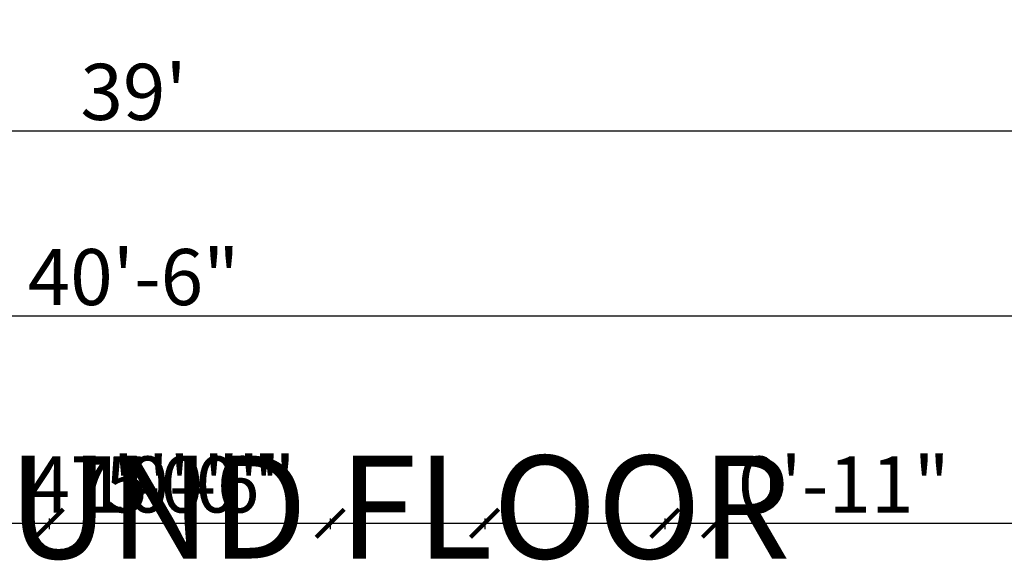
# Model space of a CAD drawing. Units: inches. Extents: x 261 to 2725, y 291 to 1454.
# Tile 7 of 35: x 688 to 898, y 296 to 412. Entities that reach past the tile are written whole.
import ezdxf

# ---------------------------------------------------------------- set-up
doc = ezdxf.new("R2010")
doc.units = ezdxf.units.IN
doc.layers.add('A-ANNO-DIMS', color=136, linetype='Continuous', lineweight=18)
doc.layers.add('A-ANNO-TEXT', color=7, linetype='Continuous', lineweight=25)
doc.styles.get("Standard").update_dxf_attribs({"font": 'arial.ttf'})
doc.dimstyles.new('ISO-25', dxfattribs={"dimtxt": 12, "dimasz": 6, "dimexe": 1.25, "dimexo": 0.625, "dimtad": 1, "dimdec": 0, "dimlunit": 3, "dimtxsty": 'Standard', "dimblk": 'ARCHTICK', "dimcen": 2.5, "dimadec": 0, "dimazin": 0, "dimtfac": 1, "dimtdec": 0, "dimtmove": 0, "dimatfit": 3, "dimfxl": 1, "dimfxlon": 1, "dimarcsym": 0})

# ---------------------------------------------------------------- blocks, each defined once
blk = doc.blocks.new('_ArchTick')
at = {"color": 0, "linetype": 'ByBlock', "const_width": 0.15}
blk.add_lwpolyline([(-0.5, -0.5), (0.5, 0.5)], dxfattribs=at)
blk = doc.blocks.new('*D28')
at = {"layer": 'A-ANNO-DIMS', "color": 0, "lineweight": -2, "transparency": 16777216}
for p, q in [((469.45, 349.55), (469.45, 347.3)), ((955.45, 349.55), (955.45, 347.3)), ((469.45, 348.55), (955.45, 348.55))]:
    blk.add_line(p, q, dxfattribs=at)
at = {"layer": 'Defpoints', "color": 0, "transparency": 16777216}
for p in [(469.45, 508.47), (955.45, 508.47), (955.45, 348.55)]:
    blk.add_point(p, dxfattribs=at)
at = {"layer": 'A-ANNO-DIMS', "color": 0, "lineweight": -2, "transparency": 16777216, "xscale": 6, "yscale": 6, "zscale": 6, "rotation": 180}
blk.add_blockref('_ArchTick', (469.45, 348.55), dxfattribs=at)
at = {"layer": 'A-ANNO-DIMS', "color": 0, "lineweight": -2, "transparency": 16777216, "xscale": 6, "yscale": 6, "zscale": 6}
blk.add_blockref('_ArchTick', (955.45, 348.55), dxfattribs=at)
at = {"layer": 'A-ANNO-DIMS', "color": 0, "transparency": 16777216, "insert": (712.45, 355.3), "char_height": 12, "attachment_point": 5}
blk.add_mtext('40\'-6"', dxfattribs=at)
blk = doc.blocks.new('*D31')
at = {"layer": 'A-ANNO-DIMS', "color": 0, "lineweight": -2, "transparency": 16777216}
for p, q in [((478.45, 389.14), (478.45, 386.89)), ((946.45, 389.14), (946.45, 386.89)), ((478.45, 388.14), (946.45, 388.14))]:
    blk.add_line(p, q, dxfattribs=at)
at = {"layer": 'Defpoints', "color": 0, "transparency": 16777216}
for p in [(478.45, 517.47), (946.45, 517.47), (946.45, 388.14)]:
    blk.add_point(p, dxfattribs=at)
at = {"layer": 'A-ANNO-DIMS', "color": 0, "lineweight": -2, "transparency": 16777216, "xscale": 6, "yscale": 6, "zscale": 6, "rotation": 180}
blk.add_blockref('_ArchTick', (478.45, 388.14), dxfattribs=at)
at = {"layer": 'A-ANNO-DIMS', "color": 0, "lineweight": -2, "transparency": 16777216, "xscale": 6, "yscale": 6, "zscale": 6}
blk.add_blockref('_ArchTick', (946.45, 388.14), dxfattribs=at)
at = {"layer": 'A-ANNO-DIMS', "color": 0, "transparency": 16777216, "insert": (712.45, 394.89), "char_height": 12, "attachment_point": 5}
blk.add_mtext("39'", dxfattribs=at)
blk = doc.blocks.new('*D87')
at = {"layer": 'A-ANNO-DIMS', "color": 0, "lineweight": -2, "ltscale": 0.07, "transparency": 16777216}
for p, q in [((694.45, 305.22), (694.45, 302.97)), ((754.45, 305.22), (754.45, 302.97)), ((694.45, 304.22), (754.45, 304.22))]:
    blk.add_line(p, q, dxfattribs=at)
at = {"layer": 'Defpoints', "color": 0, "ltscale": 0.07, "transparency": 16777216}
for p in [(694.45, 508.47), (754.45, 508.47), (754.45, 304.22)]:
    blk.add_point(p, dxfattribs=at)
at = {"layer": 'A-ANNO-DIMS', "color": 0, "lineweight": -2, "ltscale": 0.07, "transparency": 16777216, "xscale": 6, "yscale": 6, "zscale": 6, "rotation": 180}
blk.add_blockref('_ArchTick', (694.45, 304.22), dxfattribs=at)
at = {"layer": 'A-ANNO-DIMS', "color": 0, "lineweight": -2, "ltscale": 0.07, "transparency": 16777216, "xscale": 6, "yscale": 6, "zscale": 6}
blk.add_blockref('_ArchTick', (754.45, 304.22), dxfattribs=at)
at = {"layer": 'A-ANNO-DIMS', "color": 0, "ltscale": 0.07, "transparency": 16777216, "insert": (724.45, 310.97), "char_height": 12, "attachment_point": 5}
blk.add_mtext('5\'-0"', dxfattribs=at)
blk = doc.blocks.new('*D88')
at = {"layer": 'A-ANNO-DIMS', "color": 0, "lineweight": -2, "ltscale": 0.07, "transparency": 16777216}
for p, q in [((430.45, 305.22), (430.45, 302.97)), ((994.45, 305.22), (994.45, 302.97)), ((430.45, 304.22), (994.45, 304.22))]:
    blk.add_line(p, q, dxfattribs=at)
at = {"layer": 'Defpoints', "color": 0, "ltscale": 0.07, "transparency": 16777216}
for p in [(430.45, 412.47), (994.45, 412.47), (994.45, 304.22)]:
    blk.add_point(p, dxfattribs=at)
at = {"layer": 'A-ANNO-DIMS', "color": 0, "lineweight": -2, "ltscale": 0.07, "transparency": 16777216, "xscale": 6, "yscale": 6, "zscale": 6, "rotation": 180}
blk.add_blockref('_ArchTick', (430.45, 304.22), dxfattribs=at)
at = {"layer": 'A-ANNO-DIMS', "color": 0, "lineweight": -2, "ltscale": 0.07, "transparency": 16777216, "xscale": 6, "yscale": 6, "zscale": 6}
blk.add_blockref('_ArchTick', (994.45, 304.22), dxfattribs=at)
at = {"layer": 'A-ANNO-DIMS', "color": 0, "ltscale": 0.07, "transparency": 16777216, "insert": (712.45, 310.97), "char_height": 12, "attachment_point": 5}
blk.add_mtext('47\'-0"', dxfattribs=at)
blk = doc.blocks.new('*D93')
at = {"layer": 'A-ANNO-DIMS', "color": 0, "lineweight": -2, "ltscale": 0.07, "transparency": 16777216}
for p, q in [((661.45, 305.22), (661.45, 302.97)), ((787.45, 305.22), (787.45, 302.97)), ((661.45, 304.22), (787.45, 304.22))]:
    blk.add_line(p, q, dxfattribs=at)
at = {"layer": 'Defpoints', "color": 0, "ltscale": 0.07, "transparency": 16777216}
for p in [(661.45, 430.47), (787.45, 430.47), (787.45, 304.22)]:
    blk.add_point(p, dxfattribs=at)
at = {"layer": 'A-ANNO-DIMS', "color": 0, "lineweight": -2, "ltscale": 0.07, "transparency": 16777216, "xscale": 6, "yscale": 6, "zscale": 6, "rotation": 180}
blk.add_blockref('_ArchTick', (661.45, 304.22), dxfattribs=at)
at = {"layer": 'A-ANNO-DIMS', "color": 0, "lineweight": -2, "ltscale": 0.07, "transparency": 16777216, "xscale": 6, "yscale": 6, "zscale": 6}
blk.add_blockref('_ArchTick', (787.45, 304.22), dxfattribs=at)
at = {"layer": 'A-ANNO-DIMS', "color": 0, "ltscale": 0.07, "transparency": 16777216, "insert": (724.45, 310.97), "char_height": 12, "attachment_point": 5}
blk.add_mtext('10\'-6"', dxfattribs=at)
blk = doc.blocks.new('*D99')
at = {"layer": 'A-ANNO-DIMS', "color": 0, "lineweight": -2, "ltscale": 0.07, "transparency": 16777216}
for p, q in [((825.95, 305.22), (825.95, 302.97)), ((836.95, 305.22), (836.95, 302.97)), ((825.95, 304.22), (836.95, 304.22)), ((836.95, 304.22), (885.42, 304.22))]:
    blk.add_line(p, q, dxfattribs=at)
at = {"layer": 'Defpoints', "color": 0, "ltscale": 0.07, "transparency": 16777216}
for p in [(825.95, 679.47), (836.95, 679.47), (836.95, 304.22)]:
    blk.add_point(p, dxfattribs=at)
at = {"layer": 'A-ANNO-DIMS', "color": 0, "lineweight": -2, "ltscale": 0.07, "transparency": 16777216, "xscale": 6, "yscale": 6, "zscale": 6, "rotation": 180}
blk.add_blockref('_ArchTick', (825.95, 304.22), dxfattribs=at)
at = {"layer": 'A-ANNO-DIMS', "color": 0, "lineweight": -2, "ltscale": 0.07, "transparency": 16777216, "xscale": 6, "yscale": 6, "zscale": 6}
blk.add_blockref('_ArchTick', (836.95, 304.22), dxfattribs=at)
at = {"layer": 'A-ANNO-DIMS', "color": 0, "ltscale": 0.07, "transparency": 16777216, "insert": (864.19, 310.97), "char_height": 12, "attachment_point": 5}
blk.add_mtext('0\'-11"', dxfattribs=at)

msp = doc.modelspace()

# ---------------------------------------------------------------- texts
at = {"layer": 'A-ANNO-TEXT', "insert": (607.81, 318.69), "char_height": 22, "attachment_point": 1}
msp.add_mtext_dynamic_manual_height_columns('\\pxqc;{\\fTimes New Roman|b0|i0|c0|p18;GROUND FLOOR}', width=260.751, gutter_width=12.5, heights=[0], dxfattribs=at)

# ---------------------------------------------------------------- dimensions: what is measured, and where the dimension line sits
at = {"layer": 'A-ANNO-DIMS', "ltscale": 0.07}
for base, p1, p2, picture, middle in [((836.95, 304.22), (825.95, 679.47), (836.95, 679.47), '*D99', (864.19, 310.97)), ((754.45, 304.22), (694.45, 508.47), (754.45, 508.47), '*D87', (724.45, 310.97)), ((787.45, 304.22), (661.45, 430.47), (787.45, 430.47), '*D93', (724.45, 310.97)), ((994.45, 304.22), (430.45, 412.47), (994.45, 412.47), '*D88', (712.45, 310.97))]:
    dim = msp.add_linear_dim(base=base, p1=p1, p2=p2, dimstyle='ISO-25', override={"dimdec": 1, "dimlfac": 1, "dimrnd": 0, "dimzin": 1, "dimdsep": 46, "dimlunit": 4, "dimfrac": 2}, dxfattribs=at)
    dim.commit()
    dim.dimension.update_dxf_attribs({"geometry": picture, "text_midpoint": middle})
at = {"layer": 'A-ANNO-DIMS'}
for base, p1, p2, picture, middle in [((946.45, 388.14), (478.45, 517.47), (946.45, 517.47), '*D31', (712.45, 388.14)), ((955.45, 348.55), (469.45, 508.47), (955.45, 508.47), '*D28', (712.45, 348.55))]:
    dim = msp.add_linear_dim(base=base, p1=p1, p2=p2, dimstyle='ISO-25', override={"dimclrd": 0, "dimclre": 0, "dimclrt": 0}, dxfattribs=at)
    dim.commit()
    dim.dimension.update_dxf_attribs({"geometry": picture, "text_midpoint": middle, "dimtype": 160})

doc.saveas('drawing.dxf')
